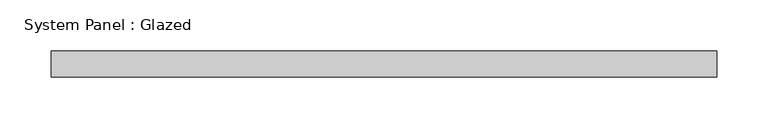
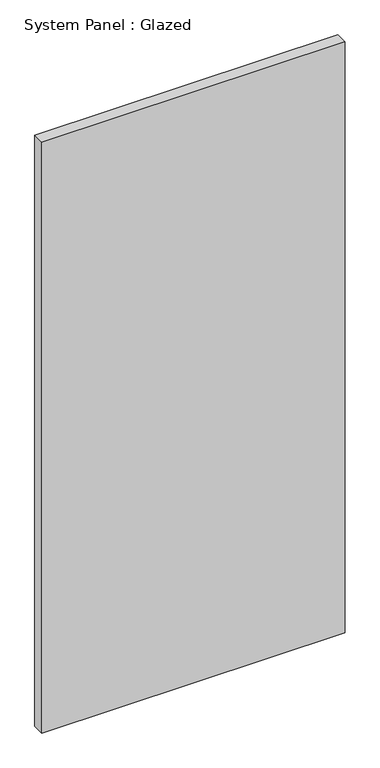
"""IFC4 building model written with IfcOpenShell, lengths in millimetres: plate geometry, System Panel : Glazed."""

from ifc_helpers import new_model, si_unit, origin, origin_with_axes, place, context, project, spatial, polyline, outline, extrude, source, transform, mapped, element, save


def system_panel_glazed_ad4bb790(model_context):
    return source(origin(), model_context, "Body", "SweptSolid", [
        extrude(outline(polyline([(323.85, 19.05), (-323.85, 19.05), (-323.85, 44.45), (323.85, 44.45), (323.85, 19.05)])), origin_with_axes(), (0.0, 0.0, 1.0), 1332.9491558),
    ])


if __name__ == "__main__":
    model = new_model("IFC4")
    model_context = context("Model", 3, world=origin())
    ifc_project = project(units=[si_unit("LENGTHUNIT", "METRE", prefix="MILLI")], contexts=[model_context])
    site = spatial("IfcSite", under=ifc_project)
    building = spatial("IfcBuilding", under=site)
    placement = place(None, origin())
    system_panel_glazed_shape = system_panel_glazed_ad4bb790(model_context)
    element("IfcPlate", 1, ObjectType="System Panel : Glazed", at=placement, inside=building, context=model_context, shape_type="MappedRepresentation", body=[
        mapped(system_panel_glazed_shape, transform((0.0, 0.0, 0.0), x_axis=(1.0, 0.0, 0.0), y_axis=(0.0, 1.0, 0.0), z_axis=(0.0, 0.0, 1.0))),
    ])
    save(model, "model.ifc")

# Revit data of these elements
# Type "System Panel : Glazed"
#   Construction Type Id = "GSP4R"
#   Analytic Construction = "1/8 in Pilkington single glazing"
#   Visual Light Transmittance = 0.9
#   Solar Heat Gain Coefficient = 0.86
#   Heat Transfer Coefficient (U) = 1.18115 BTU/(h·ft²·°F)
#   Define Thermal Properties by = 1
# Element 1 (IfcPlate, "System Panel : Glazed")
#   Materials on its faces: "Glass"
# Materials
#   "Glass": class "Glass", colour RGB 0 128 192, transparency 0.75, Description = "Soda Lime Glass", Cost = 0
